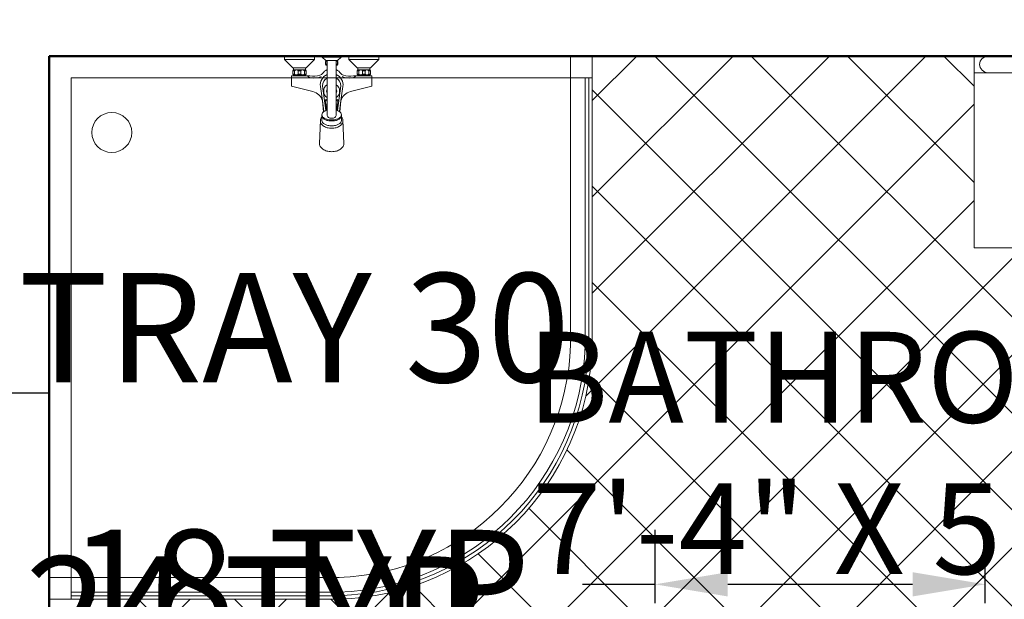
# Model space of a CAD drawing. Units: inches. Extents: x -466983 to 1020, y 324 to 318697.
# Tile 5 of 97: x 450 to 504, y 597 to 629. Entities that reach past the tile are written whole.
import ezdxf

# ---------------------------------------------------------------- set-up
doc = ezdxf.new("R2010")
doc.units = ezdxf.units.IN
doc.header["$MEASUREMENT"] = 0
for name, color, linetype, lineweight in [('A-ANNO-DIMS', 2, 'Continuous', 18), ('A-AREA-IDEN', 7, 'Continuous', 25), ('A-FLOR-FIXT', 9, 'Continuous', 18), ('A-FLOR-PATT', 252, 'Continuous', 13), ('A-GLAZ', 4, 'Continuous', 25), ('A-WALL', 7, 'Continuous', 50)]:
    doc.layers.add(name, color=color, linetype=linetype, lineweight=lineweight)
doc.styles.get("Standard").update_dxf_attribs({"font": 'arial.ttf'})
doc.dimstyles.get("Standard").update_dxf_attribs({"dimtxt": 6, "dimasz": 4, "dimexe": 3, "dimexo": 3, "dimgap": 0.09, "dimtad": 0, "dimtih": 1, "dimtoh": 1, "dimdec": 1, "dimzin": 0, "dimdsep": 46, "dimlunit": 3, "dimtxsty": 'Standard', "dimcen": 0.09, "dimadec": 0, "dimazin": 0, "dimtfac": 1, "dimtdec": 1, "dimtofl": 0, "dimtmove": 0, "dimatfit": 3, "dimfxl": 1, "dimtolj": 1, "dimtzin": 0, "dimarcsym": 0})

# ---------------------------------------------------------------- blocks, each defined once
blk = doc.blocks.new('Ventilator')
for p, q in [((1433.5927409432, 801.6799676286266), (1457.592740943201, 801.6799676286266)), ((1433.5927409432, 792.6799676286266), (1433.5927409432, 801.6799676286266)), ((1457.592740943201, 801.6799676286266), (1457.592740943201, 792.6799676286266)), ((1433.5927409432, 797.9799676286265), (1457.592740943201, 797.9799676286265)), ((1457.592740943201, 796.3799676286266), (1433.5927409432, 796.3799676286266)), ((1457.592740943201, 792.6799676286266), (1433.5927409432, 792.6799676286266))]:
    blk.add_line(p, q)
blk = doc.blocks.new('B1')
for p, q in [((0, 1300.000000000277), (693.3333333334303, 1300.000000000277)), ((0, 1.023182e-10), (0, 1300.000000000277)), ((52.00000000000727, 52.00000000000045), (52.00000000000727, 1300.000000000277)), ((52.00000000000727, 1291.33333333362), (693.3333333334303, 1291.33333333362)), ((52.00000000000727, 1282.666666666948), (693.3333333334303, 1282.666666666948)), ((0, 1248.000000000277), (693.3333333334303, 1248.000000000277)), ((21.99999999999818, 689.0000000001346), (21.99999999999818, 687.0000000001382)), ((140.3876720592416, 699.4289321882679), (154.4144116848583, 699.4289321882679)), ((208.8876720592416, 705.4289321882679), (153.4804125083301, 702.8756022550479)), ((1248.000000000174, 693.6609680139231), (1248.000000000174, 1.023182e-10)), ((1282.666666666846, 693.6609680139231), (1282.666666666846, 52.00000000010231)), ((1291.333333333514, 693.6609680139231), (1291.333333333517, 52.00000000010231)), ((1300.000000000182, 693.6609680139231), (1300.000000000182, 1.023182e-10)), ((21.99999999999818, 663.0000000001382), (21.99999999999818, 665.0000000001309)), ((140.3876720592416, 652.5710678120049), (154.4144116848583, 652.5710678120049)), ((208.8876720592416, 646.5710678120049), (153.5459520445456, 648.976381547378)), ((52.00000000001091, 52.00000000000045), (1300.000000000178, 52.00000000010231)), ((0, 4.547e-13), (1300.000000000182, 1.023182e-10))]:
    blk.add_line(p, q)
for points in [[(0, 775.000000000131), (0, 789.0000000001346), (8, 789.0000000001346)], [(8, 789.0000000001346), (8, 717.0000000001309)], [(8, 789.0000000001346), (27.99999999999818, 769.0000000001309), (27.99999999999818, 767.0000000001382)], [(0, 754.0000000001382), (0, 775.000000000131)], [(27.99999999999818, 767.0000000001382), (33.00000000000182, 767.0000000001382)], [(27.99999999999818, 767.0000000001382), (27.99999999999818, 753.0000000001345)], [(33.00000000000182, 767.0000000001382), (35, 769.0000000001309), (43, 769.0000000001309), (45.00000000000182, 767.0000000001382)], [(33.00000000000182, 767.0000000001382), (33.00000000000182, 753.0000000001345)], [(35, 765.0000000001345), (33.00000000000182, 762.0000000001346)], [(33.00000000000182, 758.0000000001346), (35, 756.0000000001346), (43, 756.0000000001346), (45.00000000000182, 758.0000000001346)], [(43, 769.0000000001309), (43, 765.0000000001345), (35, 765.0000000001345), (35, 769.0000000001309)], [(35, 756.0000000001346), (35, 753.0000000001345)], [(43, 765.0000000001345), (45.00000000000182, 763.0000000001382)], [(43, 756.0000000001346), (43, 753.0000000001345)], [(47, 767.0000000001382), (45.00000000000182, 767.0000000001382)], [(45.00000000000182, 767.0000000001382), (45.00000000000182, 753.0000000001345)], [(47, 739.0000000001382), (47, 767.0000000001382)], [(8, 717.0000000001309), (0, 717.0000000001309), (0, 754.0000000001382)], [(8, 717.0000000001309), (27.99999999999818, 737.0000000001346), (27.99999999999818, 739.0000000001382)], [(27.99999999999818, 739.0000000001382), (27.99999999999818, 753.0000000001345)], [(27.99999999999818, 739.0000000001382), (33.00000000000182, 739.0000000001382)], [(33.00000000000182, 739.0000000001382), (33.00000000000182, 753.0000000001345)], [(33.00000000000182, 748.0000000001382), (35, 750.0000000001346), (43, 750.0000000001346), (45.00000000000182, 748.0000000001382)], [(35, 741.0000000001346), (33.00000000000182, 744.0000000001345)], [(33.00000000000182, 739.0000000001382), (35, 737.0000000001346), (43, 737.0000000001346), (45.00000000000182, 739.0000000001382)], [(35, 750.0000000001346), (35, 753.0000000001345)], [(43, 737.0000000001346), (43, 741.0000000001346), (35, 741.0000000001346), (35, 737.0000000001346)], [(43, 750.0000000001346), (43, 753.0000000001345)], [(43, 741.0000000001346), (45.00000000000182, 743.0000000001346)], [(45.00000000000182, 739.0000000001382), (45.00000000000182, 753.0000000001345)], [(47, 739.0000000001382), (45.00000000000182, 739.0000000001382)], [(47, 728.0000000001345), (47, 739.0000000001382)], [(0, 687.0000000001382), (0, 699.0000000001382)], [(0, 699.0000000001382), (3, 699.0000000001382)], [(0, 665.0000000001309), (0, 687.0000000001382)], [(3, 699.0000000001382), (3, 676.0000000001346)], [(3, 699.0000000001382), (11, 690.0000000001382), (11, 687.0000000001382)], [(11, 687.0000000001382), (11, 676.0000000001346)], [(140.9999999999982, 687.0000000001382), (11, 687.0000000001382)], [(0, 653.0000000001309), (0, 665.0000000001309)], [(3, 653.0000000001309), (3, 676.0000000001346)], [(3, 653.0000000001309), (11, 662.000000000131), (11, 665.0000000001309)], [(11, 665.0000000001309), (11, 676.0000000001346)], [(140.9999999999982, 665.0000000001309), (11, 665.0000000001309)], [(0, 653.0000000001309), (3, 653.0000000001309)], [(133.9221670278657, 656.0563042479444), (133.0620831697051, 656.0563042479444)], [(7.999999999998181, 635.0000000001382), (0, 635.0000000001382), (0, 598.0000000001309)], [(7.999999999998181, 563.0000000001346), (7.999999999998181, 635.0000000001382)], [(7.999999999998181, 635.0000000001382), (27.99999999999818, 615.0000000001345), (27.99999999999818, 613.0000000001346)], [(27.99999999999818, 613.0000000001346), (27.99999999999818, 599.0000000001382)], [(27.99999999999818, 613.0000000001346), (33.00000000000182, 613.0000000001346)], [(33.00000000000182, 613.0000000001346), (35, 615.0000000001345), (42.99999999999818, 615.0000000001345), (45.00000000000182, 613.0000000001346)], [(33.00000000000182, 613.0000000001346), (33.00000000000182, 599.0000000001382)], [(42.99999999999818, 615.0000000001345), (42.99999999999818, 611.0000000001382), (35, 611.0000000001382), (35, 615.0000000001345)], [(45.00000000000182, 613.0000000001346), (45.00000000000182, 599.0000000001382)], [(47, 613.0000000001346), (45.00000000000182, 613.0000000001346)], [(47, 624.0000000001345), (47, 613.0000000001346)], [(47, 613.0000000001346), (47, 585.0000000001346)], [(0, 598.0000000001309), (0, 577.0000000001382)], [(27.99999999999818, 585.0000000001346), (27.99999999999818, 599.0000000001382)], [(35, 611.0000000001382), (33.00000000000182, 608.0000000001382)], [(33.00000000000182, 604.0000000001346), (35, 602.0000000001382), (42.99999999999818, 602.0000000001382), (45.00000000000182, 604.0000000001346)], [(33.00000000000182, 585.0000000001346), (33.00000000000182, 599.0000000001382)], [(33.00000000000182, 594.0000000001345), (35, 596.0000000001382), (42.99999999999818, 596.0000000001382), (45.00000000000182, 594.0000000001345)], [(35, 587.0000000001382), (33.00000000000182, 590.0000000001382)], [(35, 602.0000000001382), (35, 599.0000000001382)], [(35, 596.0000000001382), (35, 599.0000000001382)], [(42.99999999999818, 611.0000000001382), (45.00000000000182, 609.0000000001346)], [(42.99999999999818, 602.0000000001382), (42.99999999999818, 599.0000000001382)], [(42.99999999999818, 596.0000000001382), (42.99999999999818, 599.0000000001382)], [(45.00000000000182, 585.0000000001346), (45.00000000000182, 599.0000000001382)], [(0, 577.0000000001382), (0, 563.0000000001346), (7.999999999998181, 563.0000000001346)], [(7.999999999998181, 563.0000000001346), (27.99999999999818, 583.000000000131), (27.99999999999818, 585.0000000001346)], [(27.99999999999818, 585.0000000001346), (33.00000000000182, 585.0000000001346)], [(33.00000000000182, 585.0000000001346), (35, 583.000000000131), (42.99999999999818, 583.000000000131), (45.00000000000182, 585.0000000001346)], [(42.99999999999818, 583.000000000131), (42.99999999999818, 587.0000000001382), (35, 587.0000000001382), (35, 583.000000000131)], [(42.99999999999818, 587.0000000001382), (45.00000000000182, 589.0000000001309)], [(47, 585.0000000001346), (45.00000000000182, 585.0000000001346)]]:
    blk.add_lwpolyline(points)
blk.add_lwpolyline([(208.8876720592416, 646.5710678120049), (154.6376720593016, 648.9289321882679, -0.1383183006310921), (148.063043746286, 650.7831906028294, -0.0370381408635636), (145.578855038857, 652.5710678120049), (140.3876720592379, 652.5710678120049, -0.1665558057867227), (136.092755137337, 654.0425753596318, -0.0535717192020755), (133.4948936773198, 656.547585930646), (107, 654.0000000001382, 0.2625940722123521), (85, 631.0000000001346), (72, 580.0000000001419), (47, 580.0000000001419), (47, 585.0000000001346), (45.00000000000182, 585.0000000001346), (42.99999999999818, 583.0000000001346), (35, 583.0000000001346), (33.00000000000182, 585.0000000001346), (27.99999999999818, 585.0000000001346), (27.99999999999818, 583.0000000001346), (7.999999999998181, 563.0000000001382), (0, 563.0000000001382), (0, 577.0000000001418), (0, 598.0000000001346), (0, 635.0000000001418), (7.999999999998181, 635.0000000001418), (27.99999999999818, 615.0000000001382), (27.99999999999818, 613.0000000001346), (33.00000000000182, 613.0000000001346), (35, 615.0000000001382), (42.99999999999818, 615.0000000001382), (45.00000000000182, 613.0000000001346), (47, 613.0000000001346), (47, 624.0000000001382, 0.1247866838288863), (46, 648.0000000001382, 0.1501483781683498), (42.00000000000182, 654.0000000001382, -0.1384844099870248), (32.50754085593508, 665.0000000001345), (21.99999999999818, 665.0000000001345), (21.99999999999818, 663.0000000001382, -0.3003468456066685), (11, 662.3397459768711), (11, 662.0000000001346), (3, 653.0000000001345), (0, 653.0000000001345), (0, 665.0000000001345), (0, 687.0000000001382), (0, 699.0000000001418), (3, 699.0000000001418), (11, 690.0000000001382), (10.99999999999636, 689.6602540496569, -0.3003468456580443), (21.99999999999818, 689.0000000001346), (21.99999999999818, 687.0000000001382), (32.50754085593508, 687.0000000001382, -0.138484409987018), (42.00000000000182, 698.0000000001346, 0.1501483781683498), (46, 704.0000000001346, 0.1247866838288863), (47, 728.0000000001382), (47, 739.0000000001382), (45.00000000000182, 739.0000000001382), (43, 737.0000000001382), (35, 737.0000000001382), (33.00000000000182, 739.0000000001382), (27.99999999999818, 739.0000000001382), (27.99999999999818, 737.0000000001382), (8, 717.0000000001346), (0, 717.0000000001346), (0, 754.0000000001382), (0, 775.0000000001346), (0, 789.0000000001382), (8, 789.0000000001382), (27.99999999999818, 769.0000000001345), (27.99999999999818, 767.0000000001382), (33.00000000000182, 767.0000000001382), (35, 769.0000000001345), (43, 769.0000000001345), (45.00000000000182, 767.0000000001382), (47, 767.0000000001382), (47, 772.0000000001346), (72, 772.0000000001346), (85, 721.0000000001382, 0.2625940722123521), (107, 698.0000000001346), (133.494893670435, 695.4524140702815, -0.0535717192022979), (136.092755137337, 697.9574246406409, -0.1665558057868109), (140.3876720592416, 699.4289321882679), (145.7502000114491, 699.4289321882679, -0.0343443404771406), (148.063043746286, 701.07467377371, -0.1383183006298331), (154.6376720592416, 702.9289321882715), (208.8876720591488, 705.4289321882679, -0.1377032461334603), (216.0999264221609, 703.4042378869926, -0.1070360850488126), (223.0298076829695, 696.809397513447, -0.0808015121757586), (227.273223711496, 687.6931912444343, -0.0687078013104136), (228.8876720592398, 676.0000000001382, -0.0687078013104135), (227.273223711496, 664.3068087558385, -0.0808015121757595), (223.0298076829695, 655.1906024868258, -0.107036085048811), (216.0999264221609, 648.5957621132802, -0.1377032461317454)], format="xyb", close=True)
for points in [[(47, 767.0000000001382), (47, 772.0000000001309), (72, 772.0000000001309), (85, 721.0000000001382, 0.2625940722123521), (107, 698.0000000001346), (133.4948936704422, 695.4524140702887, -0.3591123035969264)], [(47, 734.0000000001346, -0.2052577019546359), (52, 726.0000000001309, -0.1374236490949136), (49, 701.0000000001346, -5.029096516974528)], [(47, 728.0000000001345, -0.1247866838288863), (46, 704.0000000001346, -0.1501483781683498), (42.00000000000182, 698.0000000001346, 0.138484409987018), (32.50754085593508, 687.0000000001382, 0.7633705308853952)], [(11, 688.0000000001346, -0.2034527507076884), (11.27314869702968, 688.6434964536201, -0.0971632324952149), (12.46446609406666, 689.4142135625043, -0.0541309211895364), (13.96123847455419, 689.8322469457524, -0.041071521782227), (15.99999999999818, 690.0000000001382, -0.041071521782232), (18.03876152544581, 689.8322469457524, -0.0541309211895581), (19.53553390593333, 689.4142135625043, -0.0971632324952149), (20.72685130297032, 688.6434964536201, -0.2034527507076884), (21, 688.0000000001346, -0.2034527507076693), (20.72685130297032, 687.3565035466526, -0.0379533313060429), (20.29672106629732, 687.0000000001382, -0.0541309211895384)], [(11.70327893370086, 687.0000000001382, -0.0379533313059558), (11.27314869702968, 687.3565035466526, -0.2034527507076722), (11, 688.0000000001346, -0.2034527507076884)], [(11.14357068821118, 689.7415727613479, -0.2958552022276962), (21.99999999999818, 689.0000000001346, -2.290285352134018)], [(106.0000000000018, 698.0000000001346), (73, 703.0000000001382, 0.3410628393219512), (44.19402075297876, 687.0000000001382, 0.987420997957196)], [(71.00000000000182, 698.0000000001346, 0.2653451188970793), (52.73167562087656, 687.0000000001382, 0.6855978624637613)], [(71.00000000000182, 698.0000000001346), (130.3767751999166, 690.0830966401517, -0.389881551935721)], [(109.0000000000018, 693.0000000001382, 0.3394066855219726), (103.0542662941007, 687.0000000001382)], [(105.3371881863113, 687.0000000001382, -0.2701562118716146), (110, 691.0000000001346), (129.6983785438242, 688.2641140912746, -0.3982822486971544)], [(106.0000000000018, 698.0000000001346), (132.9051195245556, 694.7054955685562, -0.3445125279727503)], [(129.2869436463206, 665.0799945585786, 0.0546118951167688), (131.5488372944073, 659.4332431739494, 0.1055200220071626), (136.092755137337, 654.0425753596318, 0.1665558057868128), (140.3876720592416, 652.5710678120049, 0.1665558057868108), (144.6825889811407, 654.0425753596318, 0.1055200220071628), (149.2265068240704, 659.4332431739494, 0.0682582856346859), (151.8562849435693, 666.5533485092964, 0.0544283700167335), (152.8876720592398, 676.0000000001346, 0.0544283700167333), (151.8562849435693, 685.4466514909764, 0.0682582856346864), (149.2265068240704, 692.5667568263307, 0.1055200220071624), (144.6825889811407, 697.9574246406409, 0.1665558057868127), (140.3876720592416, 699.4289321882679, 0.1665558057868109), (136.092755137337, 697.9574246406409, 0.1055200220071607), (131.5488372944073, 692.5667568263307, 0.0538660454735237), (129.3093729212014, 687.0000000001382, 0.0544283700167342)], [(140.9999999999982, 665.0000000001309, 0.130158640187584), (143.919967274478, 665.7732172227988, 0.1064685849763611), (146.6568542494933, 668.2218254070867, 0.0842476149744631), (148.3593095850538, 671.6519929664936, 0.0732806852421333), (149, 676.0000000001346, 0.0732806852421325), (148.3593095850538, 680.3480070337755, 0.0842476149744645), (146.6568542494933, 683.7781745931861, 0.1064685849763632), (143.919967274478, 686.226782777474, 0.1301586401875921), (140.9999999999982, 687.0000000001382, 0.1301586401875932)], [(141.6455361051521, 652.6849517968694, 0.0451764077839428), (142.9034001510663, 652.5710678120049, 0.1665558057868108), (147.1983170729654, 654.0425753596318, 0.1055200220071628), (151.7422349158969, 659.4332431739494, 0.0682582856346859), (154.3720130353958, 666.5533485092964, 0.0544283700167335), (155.4034001510663, 676.0000000001346, 0.0544283700167333), (154.3720130353958, 685.4466514909764, 0.0682582856346864), (151.7422349158969, 692.5667568263307, 0.1055200220071624), (147.1983170729654, 697.9574246406409, 0.1665558057868127), (142.9034001510663, 699.4289321882679, 0.0451764077839423), (141.6455361051521, 699.315048203407, 0.1055200220071607)], [(145.5788550388533, 652.5710678120049, 0.0370381408635636), (148.063043746286, 650.7831906028294, 0.1383183006298338), (154.6376720592416, 648.9289321882679, 0.138318300629834), (161.2123003721917, 650.7831906028294, 0.1070627939593127), (167.5423708158942, 656.8370490962297, 0.0805227312927088), (171.4136097265637, 665.1966168081926, 0.0683531574638633), (172.8876720592398, 675.9289321882679, 0.0683531574638646), (171.4136097265637, 686.6612475683432, 0.0805227312927094), (167.5423708158942, 695.0208152803061, 0.1070627939593105), (161.2123003721917, 701.07467377371, 0.1383183006298341), (154.6376720592416, 702.9289321882715, 0.1383183006298331), (148.063043746286, 701.07467377371, 0.0343443404771406), (145.7502000114491, 699.4289321882679, 0.0805227312927093)], [(154.4144116848583, 652.5710678120049, 0.1665558057868108), (158.7093286067611, 654.0425753596318, 0.1055200220071628), (163.2532464496908, 659.4332431739494, 0.0682582856346859), (165.8830245691897, 666.5533485092964, 0.0544283700167335), (166.9144116848601, 676.0000000001346, 0.0544283700167333), (165.8830245691897, 685.4466514909764, 0.0682582856346864), (163.2532464496908, 692.5667568263307, 0.1055200220071624), (158.7093286067611, 697.9574246406409, 0.1665558057868127), (154.4144116848583, 699.4289321882679, 0.1665558057868109)], [(207.6853336958775, 646.6233249695179, 0.0217212157548433), (208.8876720592416, 646.5710678120049, 0.1377032461317454), (216.0999264221609, 648.5957621132802, 0.107036085048811), (223.0298076829695, 655.1906024868258, 0.0808015121757595), (227.273223711496, 664.3068087558385, 0.0687078013104135), (228.8876720592398, 676.0000000001346, 0.0687078013104136), (227.273223711496, 687.6931912444343, 0.0808015121757586), (223.0298076829695, 696.809397513447, 0.1070360850488126), (216.0999264221609, 703.4042378869926, 0.1377032461317515), (208.8876720592416, 705.4289321882679, 0.0115815460008583), (208.2459469633304, 705.4140658567775, 0.1070360850488107)], [(11, 664.0000000001346, 0.2034527507076884), (11.27314869702968, 663.356503546649, 0.0971632324952149), (12.46446609406666, 662.5857864377649, 0.0541309211895364), (13.96123847455419, 662.1677530545167, 0.041071521782227), (15.99999999999818, 662.000000000131, 0.041071521782232), (18.03876152544581, 662.1677530545167, 0.0541309211895581), (19.53553390593333, 662.5857864377649, 0.0971632324952149), (20.72685130297032, 663.356503546649, 0.2034527507076884), (21, 664.0000000001346, 0.2034527507076693), (20.72685130297032, 664.6434964536202, 0.0379533313062782), (20.29672106629369, 665.0000000001309, 0.0541309211895384)], [(11.70327893370449, 665.0000000001309, 0.0379533313061481), (11.27314869702968, 664.6434964536202, 0.2034527507076722), (11, 664.0000000001346, 0.2034527507076884)], [(11.14357068821118, 662.2584272389249, 0.2958552022276962), (21.99999999999818, 663.0000000001382, 2.290285352134018)], [(47, 624.0000000001345, 0.1247866838288863), (46, 648.0000000001382, 0.1501483781683498), (42.00000000000182, 654.0000000001382, -0.1384844099870248), (32.50754085593508, 665.0000000001309, -0.7633705308853952)], [(106.0000000000018, 654.0000000001382), (73, 649.0000000001345, -0.341062839321959), (44.19402075297876, 665.0000000001309, -0.987420997957196)], [(71.00000000000182, 654.0000000001382, -0.2653451188970914), (52.73167562087656, 665.0000000001309, -0.6855978624637613)], [(71.00000000000182, 654.0000000001382), (130.3767751999166, 661.9169033601211, 0.389881551935721)], [(109.0000000000018, 659.0000000001309, -0.3394066855220244), (103.0542662941007, 665.0000000001309)], [(105.3371881863113, 665.0000000001309, 0.2701562118716416), (110, 661.0000000001345), (129.6983785438278, 663.7358859089982, 0.3982822486971544)], [(47, 585.0000000001346), (47, 580.0000000001382), (72, 580.0000000001382), (85, 631.0000000001346, -0.2625940722123521), (107, 654.0000000001382), (132.4235230446356, 656.4445695236572, 0.3591123035969264)], [(47, 618.0000000001346, 0.2052577019546359), (52, 626.0000000001382, 0.1374236490949136), (49, 651.0000000001382, 5.029096516974528)], [(106.0000000000018, 654.0000000001382), (132.9051195245556, 657.2945044317166, 0.3445125279727503)]]:
    blk.add_lwpolyline(points, format="xyb")
blk.add_circle((182.931355266388, 149.5974501754249), 47.86997641275996)
for centre, radius, start, end in [((672.5535632588981, 672.5422464127919), 627.8017452838134, 1.92774542086775, 88.10320593202876), ((672.5535632588981, 672.5422464127919), 610.4684119504776, 1.92774542086775, 88.10320593202876), ((672.5535632588981, 672.5422464127919), 619.1350786171454, 1.92774542086775, 88.10320593202876), ((672.5535632588981, 672.5422464127919), 575.801745283806, 1.92774542086775, 88.10320593202876), ((84, 676.0000000001346), 19, 35.37654015188604, 144.6234598481139), ((84, 676.0000000001346), 12.00000000000001, 66.44353569094163, 113.5564643090584), ((120.8125, 676.1250000001309), 12.8131097415889, 112.0608994672246, 121.9251013585072), ((123.9999999999982, 676.0000000001346), 13, 64.79528984039216, 122.2042275039623), ((84, 676.0000000001346), 19, 215.376540151886, 324.623459848114), ((84, 676.0000000001346), 12.00000000000001, 246.4435356909416, 293.5564643090584), ((120.8125, 675.8750000001382), 12.8131097415889, 238.0748986414927, 247.9391005327754), ((123.9999999999982, 676.0000000001346), 13, 237.7957724960376, 295.2047101596079)]:
    blk.add_arc(centre, radius, start, end)
blk = doc.blocks.new('B3')
for p, q in [((-450, 0), (-455.7402514854766, -1.1418070123309)), ((450, 0), (455.7402514854766, -1.1418070123309)), ((-463.8581929876745, -9.25974851452338), (-465, -15)), ((-465, -15), (-463.8581929876745, -20.74025148547662)), ((-460.6066017178018, -4.393398282201815), (-463.8581929876745, -9.25974851452338)), ((-455.7402514854766, -1.1418070123309), (-460.6066017178018, -4.393398282201815)), ((455.7402514854766, -1.1418070123309), (460.6066017177945, -4.393398282201815)), ((460.6066017177945, -4.393398282201815), (463.8581929876672, -9.25974851452338)), ((463.8581929876672, -9.25974851452338), (465, -15)), ((465, -15), (463.8581929876672, -20.74025148547662)), ((475, -30), (-475, -30)), ((-463.8581929876745, -20.74025148547662), (-460.6066017178018, -25.60660171779819)), ((-460.6066017178018, -25.60660171779819), (-455.7402514854766, -28.8581929876691)), ((-455.7402514854766, -28.8581929876691), (-450, -30)), ((455.7402514854766, -28.8581929876691), (450, -30)), ((460.6066017177945, -25.60660171779819), (455.7402514854766, -28.8581929876691)), ((463.8581929876672, -20.74025148547662), (460.6066017177945, -25.60660171779819)), ((2.91038e-11, -182.0000000000054), (-115.8117069986983, -182.0000000000054)), ((2.91038e-11, -182.0000000000054), (115.8117069987565, -182.0000000000054))]:
    blk.add_line(p, q)
blk.add_lwpolyline([(199.4833683843535, -575, 0.2017697719241106), (217.3542190239823, -567.482353886593), (392.5, -345), (435, -345), (475, -345), (475, 0), (-475, 0), (-475, -345), (-435, -345), (-392.5, -345), (-217.3542190239896, -567.482353886593, 0.2017697719241107), (-199.4833683843608, -575)], format="xyb", close=True)
for centre, radius, start, end in [((5.09317e-11, -450.0000000000327), 400.0000000000322, 90, 119.7172288959075), ((0, -450.0000000000327), 400.0000000000319, 60.28277110409252, 90), ((2.91038e-11, -450.0000000000055), 385, 90, 111.6513567404431), ((2.91038e-11, -450.0000000000055), 385, 68.34864325955687, 90), ((-88.47222222221171, -295.0000000000055), 221.527777777762, 119.7172288959075, 240.2827711040925), ((-138.3591766736499, -101.4576952073475), 10, 111.6513567404431, 193.3915177581575), ((338.3178096717893, 12.0282100348104), 500, 193.3915177581575, 202.0594091764406), ((-338.3178096717383, 12.0282100348104), 500, 337.9405908235594, 346.6084822418425), ((138.3591766737008, -101.4576952073475), 10, 346.6084822418425, 68.34864325955687), ((88.47222222225537, -294.9999999999964), 221.527777777762, 299.7172288959074, 60.28277110409252), ((2.91038e-11, -136.9999999999891), 17.5, 90, 270), ((2.91038e-11, -136.9999999999891), 17.5, 270, 90), ((-180.5137974189128, -229.2550553338115), 64.41699441097052, 40.71477974361456, 144.4619255202982), ((-180.5137974189128, -229.2550553338115), 60.41699441097051, 40.71477974361456, 144.4619255202982), ((-115.8117069986983, -172.0000000000145), 10, 202.0594091764406, 270), ((115.8117069987565, -172.0000000000145), 10, 270, 337.9405908235594), ((180.5137974189638, -229.2550553338115), 64.41699441097052, 35.53807447970174, 139.2852202563854), ((180.5137974189638, -229.2550553338115), 60.41699441097051, 35.53807447970174, 139.2852202563854), ((-88.47222222221171, -295.0000000000055), 177.5277777777778, 144.4619255202982, 240.2827711040925), ((-88.47222222221171, -295.0000000000055), 173.5277777777778, 144.4619255202982, 240.2827711040925), ((88.47222222223354, -295.0000000000055), 173.5277777777778, 299.7172288959074, 35.53807447970174), ((88.47222222223354, -295.0000000000055), 177.5277777777778, 299.7172288959074, 35.53807447970174), ((2.91038e-11, -247.0000000000037), 37.5, 90, 270), ((2.91038e-11, -247.0000000000037), 37.5, 270, 90), ((2.91038e-11, -247.0000000000037), 23, 90, 270), ((2.91038e-11, -247.0000000000037), 23, 270, 90), ((2.91038e-11, -140.0000000000036), 356, 240.2827711040925, 270), ((2.91038e-11, -140.0000000000036), 352, 240.2827711040925, 270), ((2.91038e-11, -140.0000000000036), 352, 270, 299.7172288959074), ((2.91038e-11, -140.0000000000036), 356, 270, 299.7172288959074), ((5.09317e-11, -139.9999999999781), 400.0000000000309, 240.2827711040925, 270), ((-1.45519e-11, -140.0000000000309), 399.9999999999781, 270, 299.7172288959074)]:
    blk.add_arc(centre, radius, start, end)
blk = doc.blocks.new('*D61')
at = {"layer": 'A-ANNO-DIMS', "color": 0, "lineweight": -2, "transparency": 16777216}
for p, q in [((439.8056775209044, 608.403511460552), (436.2056775209045, 608.403511460552)), ((439.2056775209045, 604.403511460552), (439.2056775209045, 599.5978770812881)), ((439.2056775209045, 588.4035114605508), (439.2056775209045, 593.2091458398146)), ((439.8056775209044, 584.4035114605508), (436.2056775209045, 584.4035114605508))]:
    blk.add_line(p, q, dxfattribs=at)
at = {"layer": 'A-ANNO-DIMS', "color": 0, "transparency": 16777216}
for points in [[(438.5390108542378, 604.403511460552), (439.8723441875712, 604.403511460552), (439.2056775209045, 608.403511460552)], [(438.5390108542378, 588.4035114605508), (439.8723441875712, 588.4035114605508), (439.2056775209045, 584.4035114605508)]]:
    blk.add_solid(points, dxfattribs=at)
at = {"layer": 'Defpoints', "color": 0, "transparency": 16777216}
for p in [(442.8056775209045, 608.403511460552), (439.2056775209045, 584.4035114605508), (442.8056775209045, 584.4035114605508)]:
    blk.add_point(p, dxfattribs=at)
at = {"layer": 'A-ANNO-DIMS', "color": 0, "transparency": 16777216, "insert": (439.2056775209046, 596.403511460551), "char_height": 6, "attachment_point": 5}
blk.add_mtext('\\A1;VENTILATOR 24 TYP.', dxfattribs=at)
blk = doc.blocks.new('*D75')
at = {"layer": 'A-ANNO-DIMS', "color": 0, "lineweight": -2, "transparency": 16777216}
for p, q in [((448.8056775209043, 626.937732818422), (444.3217849538132, 626.937732818422)), ((447.3217849538133, 622.937732818422), (447.3217849538133, 615.1878362669078)), ((447.3217849538133, 601.0451157044797), (447.3217849538133, 608.7950122559939)), ((448.8056775209043, 597.0451157044797), (444.3217849538132, 597.0451157044797))]:
    blk.add_line(p, q, dxfattribs=at)
at = {"layer": 'A-ANNO-DIMS', "color": 0, "transparency": 16777216}
for points in [[(446.6551182871466, 622.937732818422), (447.9884516204799, 622.937732818422), (447.3217849538133, 626.937732818422)], [(446.6551182871466, 601.0451157044797), (447.9884516204799, 601.0451157044797), (447.3217849538133, 597.0451157044797)]]:
    blk.add_solid(points, dxfattribs=at)
at = {"layer": 'Defpoints', "color": 0, "transparency": 16777216}
for p in [(451.8056775209043, 626.937732818422), (447.3217849538133, 597.0451157044797), (451.8056775209043, 597.0451157044797)]:
    blk.add_point(p, dxfattribs=at)
at = {"layer": 'A-ANNO-DIMS', "color": 0, "transparency": 16777216, "insert": (447.3217849538133, 611.9914242614506), "char_height": 6, "attachment_point": 5}
blk.add_mtext('\\A1;SHOWER TRAY 30', dxfattribs=at)
blk = doc.blocks.new('*D78')
at = {"layer": 'A-ANNO-DIMS', "color": 0, "lineweight": -2, "transparency": 16777216}
for p, q in [((485.1546064346699, 596.8335263890426), (485.1546064346699, 600.8678954246358)), ((503.334059280452, 596.8335263890426), (503.334059280452, 600.8678954246358)), ((485.1546064346699, 597.8678954246357), (481.1546064346699, 597.8678954246357)), ((499.334059280452, 597.8678954246357), (489.1546064346699, 597.8678954246357))]:
    blk.add_line(p, q, dxfattribs=at)
at = {"layer": 'A-ANNO-DIMS', "color": 0, "transparency": 16777216}
for points in [[(489.1546064346699, 598.5345620913023), (489.1546064346699, 597.2012287579691), (485.1546064346699, 597.8678954246357)], [(499.334059280452, 598.5345620913023), (499.334059280452, 597.2012287579691), (503.334059280452, 597.8678954246357)]]:
    blk.add_solid(points, dxfattribs=at)
at = {"layer": 'Defpoints', "color": 0, "transparency": 16777216}
for p in [(485.1546064346699, 597.8678954246357), (485.1546064346699, 593.8335263890426), (503.334059280452, 593.8335263890426)]:
    blk.add_point(p, dxfattribs=at)
at = {"layer": 'A-ANNO-DIMS', "color": 0, "transparency": 16777216, "insert": (466.7440061618186, 597.8678954246357), "char_height": 6, "attachment_point": 5}
blk.add_mtext('\\A1;18 TYP.', dxfattribs=at)

msp = doc.modelspace()

# ---------------------------------------------------------------- hatches: boundary and pattern name
at = {"layer": 'A-FLOR-PATT', "transparency": 33554572}
h = msp.add_hatch(dxfattribs=at)
h.set_pattern_fill('ANSI37', color=256, scale=30)
h.set_pattern_definition([(45, (-1212.413693079869, -290.0350025265127), (-2.651650429449553, 2.651650429449553), []), (135, (-1212.413693079869, -290.0350025265127), (-2.651650429449553, -2.651650429449552), [])])
h.paths.add_polyline_path([(901.805677520904, 1075.937732818422), (900.6144036774049, 1075.937732818422), (900.6144036774049, 1065.385628316983), (899.390971271441, 1065.385628316983), (898.0910743401043, 1065.385628316983), (892.8355944880973, 1058.709752245277, -0.2583770168556315), (892.18750428989, 1058.350891982691), (879.9847834232776, 1058.350891982691, -0.2017697719240963), (879.438188978411, 1058.580825279484), (874.0812133730635, 1065.385628316983), (872.7813164417267, 1065.385628316983), (871.5578840357629, 1065.385628316983), (871.5578840357629, 1075.937732818422), (813.8056775209042, 1075.937732818422), (813.8056775209042, 1044.792233318721), (832.3947444543938, 1044.792233318721, -0.3947951267487684), (848.6601780212009, 1028.535584015862), (848.6601780212009, 1009.937732818421), (901.805677520904, 1009.937732818421), (901.805677520904, 1015.937732818421), (901.3056775209042, 1015.937732818421), (871.3056775209039, 1015.937732818421), (871.3056775209039, 1017.250232818421), (871.3344022102003, 1017.250232818421, -0.4014527144963572), (901.3056775209042, 1045.937732818421), (901.805677520904, 1045.937732818421)])
edge = h.paths.add_edge_path(flags=16)
edge.add_line((847.7730719745084, 1068.948588737025), (847.7730719745069, 1073.708823774771))
edge.add_arc((849.2268986539951, 1073.708823774771), 1.453826679487974, 90, 180, ccw=False)
edge.add_line((849.2268986539951, 1075.162650454259), (864.4920787886183, 1075.162650454259))
edge.add_arc((864.4920787886213, 1073.708823774771), 1.453826679487974, 0, 90.00000000012102, ccw=False)
edge.add_line((865.9459054681093, 1073.708823774771), (865.9459054681081, 1069.00351244647))
edge.add_arc((832.6447385074767, 1068.976050591752), 33.30117828385809, -20.61233806670998, 0.04724903539101888, ccw=False)
edge.add_ellipse((856.8594887213083, 1058.479989307073), major_axis=(-2.091e-13, 10.21313242340307), ratio=0.6859192225533502, start_angle=100.00884331843292, end_angle=259.9911566815624, ccw=False)
edge.add_arc((881.0742389351396, 1068.976050591752), 33.30117828385809, 180.0472490354062, 200.6123380667097, ccw=False)
h.paths.add_polyline_path([(853.145578187156, 1066.481532374271), (853.145578187156, 1066.453444752512), (853.1463399851561, 1066.453444752512, 0.4331071439582673), (852.9166149812349, 1066.684892837266), (852.9166149812349, 1066.453444752512), (853.145578187156, 1066.453444752512), (853.145578187156, 1066.481532374489), (853.088019486549, 1066.612171966583, 0.6979386910037918), (852.699540939094, 1066.453444752512), (852.7003027371272, 1066.453444752512), (852.7003027371272, 1066.481532374489), (852.9166149812349, 1067.001204630995), (852.9166149812349, 1066.684892837266, -0.3962543063594317)], flags=0)
h.paths.add_polyline_path([(861.0186747055222, 1066.481532374271), (861.0186747055222, 1066.453444752512), (861.0194365035225, 1066.453444752512, 0.4164039232557909), (860.8023624614146, 1066.684892837265), (860.8023624614146, 1066.453444752512), (861.0186747055222, 1066.453444752512), (861.0186747055222, 1066.481532374489), (860.9671752720659, 1066.605255499379, 0.7133437187663149), (860.5726374574602, 1066.453444752512), (860.5733992554934, 1066.453444752512), (860.5733992554934, 1066.481532374489), (860.8023624614146, 1067.001204630995), (860.8023624614146, 1066.684892837265, -0.3799725304814568)], flags=0)
edge = h.paths.add_edge_path(flags=0)
edge.add_spline(control_points=[(861.1298377106021, 1065.785468371534), (861.4660965533383, 1065.247811229462), (861.613385559155, 1065.016139861057), (861.9832837951076, 1064.373617117607), (862.1924105327118, 1063.944313665492), (862.5613774174725, 1063.039129539609), (862.7212131906668, 1062.56326642291), (862.9865156700853, 1061.578122280975), (863.0919804897928, 1061.068856600952), (863.2452407883674, 1060.031049745086), (863.293035446714, 1059.502522766744), (863.3294736797056, 1058.440879580113), (863.3181170778639, 1057.907777155726), (863.2366033468288, 1056.85179603536), (863.1664466211855, 1056.328931215311), (862.9695120306455, 1055.307951977375), (862.8427353108815, 1054.809852090196), (862.5365466723708, 1053.852219447362), (862.3571373353129, 1053.392702749349), (861.9514237071658, 1052.524888245794), (861.7251255454219, 1052.116609101398), (861.2330086320977, 1051.362239687588), (860.9672044472572, 1051.016170456457), (860.4047960485765, 1050.394909316517), (860.1082220871676, 1050.119734477926), (859.493696255806, 1049.64606200509), (859.1757900615103, 1049.447558762665), (858.5275631429041, 1049.129883644436), (858.197273503909, 1049.010664382187), (857.5314773710529, 1048.851811036626), (857.1959384637446, 1048.812116564677), (856.5249326641573, 1048.811967422545), (856.1893892160524, 1048.851512676201), (855.5235728169741, 1049.010066967686), (855.1932673158994, 1049.129136347874), (854.5449932971788, 1049.446513839261), (854.2270557868354, 1049.644869411481), (853.6124495619564, 1050.118254324803), (853.3158265363004, 1050.393289340464), (852.7533025914207, 1051.014284587242), (852.487431959371, 1051.360227769297), (851.9951668313728, 1052.114363776776), (851.7687869247744, 1052.522535562859), (851.3628973914427, 1053.390157753425), (851.1833939042357, 1053.849589492002), (850.8770077813263, 1054.807077270704), (850.7501277313783, 1055.30511724975), (850.5529806633081, 1056.326003473117), (850.4827147921034, 1056.848835185142), (850.4009803807432, 1057.904777820697), (850.3895122452288, 1058.437874867502), (850.425728471152, 1059.499535178563), (850.4734126571939, 1060.02808465918), (850.6264565107679, 1061.065963770327), (850.7318153592672, 1061.575279204679), (850.9969137893603, 1062.560548677974), (851.1566514873134, 1063.036487374614), (851.525433403113, 1063.94184619004), (851.7344732542367, 1064.371248757046), (852.1056260411488, 1065.016350037675), (852.2544071072941, 1065.250281998093), (852.608154630964, 1065.733465727338)], knot_values=[3.915332106759953, 3.915332106759953, 3.915332106759953, 3.915332106759953, 4.013467662305501, 4.013467662305501, 4.175531746215815, 4.175531746215815, 4.337595830126129, 4.337595830126129, 4.499659914036444, 4.499659914036444, 4.661723997946757, 4.661723997946757, 4.82378808185707, 4.82378808185707, 4.985852165767384, 4.985852165767384, 5.147916249677697, 5.147916249677697, 5.30998033358801, 5.30998033358801, 5.472044417498324, 5.472044417498324, 5.634108501408637, 5.634108501408637, 5.79617258531895, 5.79617258531895, 5.958236669229264, 5.958236669229264, 6.120300753139577, 6.120300753139577, 6.282364837049891, 6.282364837049891, 6.444428920960204, 6.444428920960204, 6.606493004870517, 6.606493004870517, 6.768557088780831, 6.768557088780831, 6.930621172691144, 6.930621172691144, 7.092685256601457, 7.092685256601457, 7.254749340511771, 7.254749340511771, 7.416813424422084, 7.416813424422084, 7.578877508332397, 7.578877508332397, 7.740941592242711, 7.740941592242711, 7.903005676153024, 7.903005676153024, 8.065069760063338, 8.065069760063338, 8.22713384397365, 8.22713384397365, 8.389197927883965, 8.389197927883965, 8.551262011794279, 8.551262011794279, 8.650370494357087, 8.650370494357087, 8.650370494357087, 8.650370494357087], degree=3, periodic=0)
edge.add_line((852.6421178657537, 1065.785468371534), (861.1298377106024, 1065.785468371534))
edge = h.paths.add_edge_path(flags=0)
edge.add_ellipse((856.8495804607978, 1057.743205248224), major_axis=(-3.1e-13, 7.792134415209829), ratio=0.6878610933899516, start_angle=0, end_angle=360)
h.paths.add_polyline_path([(848.8634419841151, 1069.389059844444), (848.863441984139, 1073.960453158315, -0.4142135623709757), (849.9538119937549, 1075.050823167924), (863.765165448898, 1075.050823167924, -0.4142135623721942), (864.8555354585106, 1073.960453158308), (864.8555354584933, 1069.389059844444, -0.3889362887010341), (864.5236837164459, 1069.026979909221, -0.0435607626104464), (849.19529372618, 1069.02697990933, -0.3889362886276668)], flags=0)
h.paths.add_polyline_path([(853.1006153779753, 1068.112209480768, -1), (852.677499999749, 1068.112209480768, -1)], flags=0)
edge = h.paths.add_edge_path(flags=0)
edge.add_ellipse((856.8594887213083, 1057.33782914961), major_axis=(7.74e-14, 2.20702192546696), ratio=0.6571642650458812, start_angle=0, end_angle=360)
h.paths.add_polyline_path([(861.0414774428674, 1068.112209480768, -1), (860.6183620646412, 1068.112209480768, -1)], flags=0)
edge = h.paths.add_edge_path()
edge.add_line((573.9536545579417, 1057.341203598636), (573.9536545579417, 1075.937732818422))
edge.add_line((573.9536545579417, 1075.937732818422), (558.7307922536265, 1075.937732818422))
edge.add_line((558.7307922536265, 1075.937732818422), (558.7307922536265, 1065.385628316983))
edge.add_line((558.7307922536265, 1065.385628316983), (557.5073598476627, 1065.385628316983))
edge.add_line((557.5073598476627, 1065.385628316983), (556.207462916326, 1065.385628316983))
edge.add_line((556.207462916326, 1065.385628316983), (550.9519830643189, 1058.709752245277))
edge.add_arc((550.3038928661116, 1059.115537236419), 0.7646452537275144, 270, 327.94831933647396, ccw=False)
edge.add_line((550.3038928661116, 1058.350891982691), (538.1011719994992, 1058.350891982691))
edge.add_arc((538.1011719994992, 1059.115537236419), 0.7646452537275137, 224.3704013916024, 270, ccw=False)
edge.add_line((537.5545775546327, 1058.580825279484), (532.1976019492852, 1065.385628316983))
edge.add_line((532.1976019492852, 1065.385628316983), (530.8977050179485, 1065.385628316983))
edge.add_line((530.8977050179485, 1065.385628316983), (529.6742726119846, 1065.385628316983))
edge.add_line((529.6742726119846, 1065.385628316983), (529.6742726119846, 1075.937732818422))
edge.add_line((529.6742726119846, 1075.937732818422), (520.8056775209042, 1075.937732818422))
edge.add_line((520.8056775209042, 1075.937732818422), (520.8056775209042, 1045.937732818422))
edge.add_line((520.8056775209042, 1045.937732818422), (521.3056775209044, 1045.937732818422))
edge.add_arc((521.3056775209042, 1015.937732818422), 30.00000000000023, 2.507490703587223, 89.99999999999977, ccw=False)
edge.add_line((551.2769528316082, 1017.250232818422), (551.3056775209045, 1017.250232818422))
edge.add_line((551.3056775209045, 1017.250232818422), (551.3056775209045, 1015.937732818422))
edge.add_line((551.3056775209045, 1015.937732818422), (520.8056775209042, 1015.937732818422))
edge.add_line((520.8056775209042, 1015.937732818422), (520.8056775209042, 1009.937732818421))
edge.add_line((520.8056775209042, 1009.937732818421), (559.1912990237018, 1010.402158339383))
edge.add_arc((559.1912990237018, 1011.855985018871), 1.453826679487974, 180, 270, ccw=False)
edge.add_line((557.7374723442138, 1011.855985018871), (557.7374723442151, 1016.561296347171))
edge.add_arc((591.0386393048469, 1016.58875820189), 33.3011782838587, 159.3876619332891, 180.0472490353913, ccw=False)
edge.add_ellipse((566.8238890910148, 1027.084819486569), major_axis=(-3.171e-13, 10.21313242340307), ratio=0.6859192225533445, start_angle=280.00884331843395, end_angle=439.99115668156304, ccw=False)
edge.add_arc((542.6091388771833, 1016.58875820189), 33.3011782838584, 0.04724903544490644, 20.612338066710322, ccw=False)
edge.add_line((575.9103058378148, 1016.61622005664), (575.910305837816, 1011.855985018871))
edge.add_arc((574.4564791583282, 1011.855985018871), 1.453826679487974, -90, 0, ccw=False)
edge.add_line((574.4564791583282, 1010.402158339383), (608.8056775209044, 1009.937732818421))
edge.add_line((608.8056775209044, 1009.937732818421), (608.8056775209044, 1041.08570985546))
edge.add_line((608.8056775209044, 1041.08570985546), (590.2179319406538, 1041.08570985546))
edge.add_arc((590.7750219589672, 1057.907380652626), 16.83089295601249, 181.9277454211679, 268.1032059320871, ccw=False)
edge = h.paths.add_edge_path()
edge.add_ellipse((494.2443328575609, 583.6203939656394), major_axis=(-2.099e-13, 10.21313242340307), ratio=0.6859192225533391, start_angle=280.0088433184392, end_angle=439.99115668155895, ccw=False)
edge.add_arc((470.0295826437295, 573.1243326809605), 33.30117828385828, 0.047249035653180727, 20.612338066711573, ccw=False)
edge.add_line((503.3307496043607, 573.1517945358311), (503.3307496043621, 568.3915594979414))
edge.add_arc((501.8769229248741, 568.3915594979414), 1.453826679487974, -90, 0, ccw=False)
edge.add_line((501.8769229248741, 566.9377328184536), (539.8056775209043, 566.9377328184218))
edge.add_line((539.8056775209043, 566.9377328184218), (539.8056775209043, 572.9377328184218))
edge.add_line((539.8056775209043, 572.9377328184218), (539.3056775209043, 572.9377328184218))
edge.add_line((539.3056775209043, 572.9377328184218), (509.3056775209042, 572.9377328184218))
edge.add_line((509.3056775209042, 572.9377328184218), (509.3056775209042, 574.2502328184218))
edge.add_line((509.3056775209042, 574.2502328184218), (509.3344022102004, 574.2502328184218))
edge.add_arc((539.3056775209043, 572.9377328184218), 30.00000000000003, 90, 177.4925092964128, ccw=False)
edge.add_line((539.3056775209043, 602.9377328184218), (539.8056775209043, 602.9377328184218))
edge.add_line((539.8056775209043, 602.9377328184218), (539.8056775209043, 626.9377328184219))
edge.add_line((539.8056775209043, 626.9377328184219), (531.7718318056131, 626.9377328184219))
edge.add_line((531.7718318056131, 626.9377328184219), (531.7718318056131, 616.3856283169836))
edge.add_line((531.7718318056131, 616.3856283169836), (530.5483993996492, 616.3856283169836))
edge.add_line((530.5483993996492, 616.3856283169836), (529.2485024683125, 616.3856283169836))
edge.add_line((529.2485024683125, 616.3856283169836), (523.7105154427977, 609.3508919826913))
edge.add_line((523.7105154427977, 609.3508919826913), (510.7766285267865, 609.3508919826913))
edge.add_line((510.7766285267865, 609.3508919826913), (505.2386415012717, 616.3856283169835))
edge.add_line((505.2386415012717, 616.3856283169835), (503.9387445699351, 616.3856283169836))
edge.add_line((503.9387445699351, 616.3856283169836), (502.7153121639711, 616.3856283169836))
edge.add_line((502.7153121639711, 616.3856283169836), (502.7153121639712, 626.9377328184219))
edge.add_line((502.7153121639712, 626.9377328184219), (481.698294634846, 626.937732818422))
edge.add_line((481.698294634846, 626.937732818422), (481.6982946348461, 610.9950036909872))
edge.add_arc((467.2703297247223, 611.4728203914133), 14.43587476556121, 271.9277454211847, 358.103205932099, ccw=False)
edge.add_line((467.7559403853078, 597.0451157044822), (451.8056775209041, 597.0451157044822))
edge.add_line((451.8056775209041, 597.0451157044822), (451.8056775209041, 584.4035114605515))
edge.add_line((451.8056775209041, 584.4035114605515), (451.8056775209043, 566.9377328184218))
edge.add_line((451.8056775209043, 566.9377328184218), (486.6117427902477, 566.9377328184536))
edge.add_arc((486.6117427902477, 568.3915594979414), 1.453826679487974, 180, 270, ccw=False)
edge.add_line((485.1579161107598, 568.3915594979414), (485.157916110761, 573.0968708261933))
edge.add_arc((518.4590830713927, 573.1243326809608), 33.3011782838585, 159.387661933289, 180.0472490354759, ccw=False)
h.paths.add_polyline_path([(836.2608886421394, 1020.732838196592), (879.8898108795202, 1020.732838196592), (879.8898108795202, 1039.390182443977), (836.2608886421394, 1039.390182443977)], flags=25)
h.paths.add_polyline_path([(549.9851009445293, 1036.749159167106), (593.6140231819099, 1036.749159167106), (593.6140231819099, 1055.406503414491), (549.9851009445293, 1055.406503414491)], flags=24)
h.paths.add_polyline_path([(475.1230325221868, 595.5958681380167), (518.7519547595675, 595.5958681380167), (518.7519547595675, 614.2532123854019), (475.1230325221868, 614.2532123854019)], flags=24)

# ---------------------------------------------------------------- linework, layer by layer
at = {"layer": 'A-WALL'}
for p, q in [((451.8056775209043, 566.937732818422), (451.8056775209041, 626.9377328184219)), ((539.8056775209043, 626.9377328184219), (451.8056775209042, 626.9377328184219))]:
    msp.add_line(p, q, dxfattribs=at)

# ---------------------------------------------------------------- block references
at = {"layer": 'A-FLOR-FIXT', "xscale": 0.0229943208568735, "yscale": 0.0229943208568735, "zscale": 0.0229943208568735, "rotation": 270}
msp.add_blockref('B1', (451.8056775209041, 626.9377328184219), dxfattribs=at)
at = {"layer": 'A-FLOR-FIXT', "xscale": 0.0305858101490967, "yscale": 0.0305858101490967, "zscale": 0.0305858101490967}
msp.add_blockref('B3', (517.2435719847921, 626.9377328184219), dxfattribs=at)
at = {"layer": 'A-GLAZ', "rotation": 270}
msp.add_blockref('Ventilator', (-349.8742901077221, 2041.996252403752), dxfattribs=at)

# ---------------------------------------------------------------- texts
at = {"layer": 'A-AREA-IDEN', "insert": (461.9844353108056, 611.7651496296038), "char_height": 5, "attachment_point": 1}
msp.add_mtext_dynamic_manual_height_columns('\\pxqc;{\\fArial|b1|i0|c0|p34;BATHROOM\\P7\'-4" X 5\'-0"}', width=69.92316986614605, gutter_width=1, heights=[0], dxfattribs=at)

# ---------------------------------------------------------------- dimensions: what is measured, and where the dimension line sits
at = {"layer": 'A-ANNO-DIMS'}
for base, p1, p2, angle, text, picture, middle in [((447.3217849538133, 597.0451157044797), (451.8056775209041, 626.9377328184218), (451.8056775209041, 597.0451157044794), 270, 'SHOWER TRAY <>', '*D75', (447.3217849538133, 611.9914242614506)), ((439.2056775209045, 584.4035114605508), (442.8056775209042, 608.4035114605517), (442.8056775209042, 584.4035114605506), 270, 'VENTILATOR <> TYP.', '*D61', (439.2056775209046, 596.403511460551)), ((485.1546064346699, 597.8678954246357), (503.334059280452, 593.8335263890426), (485.1546064346699, 593.8335263890426), 180, '<> TYP.', '*D78', (466.7440061618186, 597.8678954246357))]:
    dim = msp.add_linear_dim(base=base, p1=p1, p2=p2, angle=angle, text=text, dimstyle='Standard', override={"dimdec": 0, "dimlfac": 1, "dimrnd": 0, "dimzin": 0, "dimdsep": 46, "dimlunit": 2}, dxfattribs=at)
    dim.commit()
    dim.dimension.update_dxf_attribs({"geometry": picture, "text_midpoint": middle})

doc.saveas('drawing.dxf')
